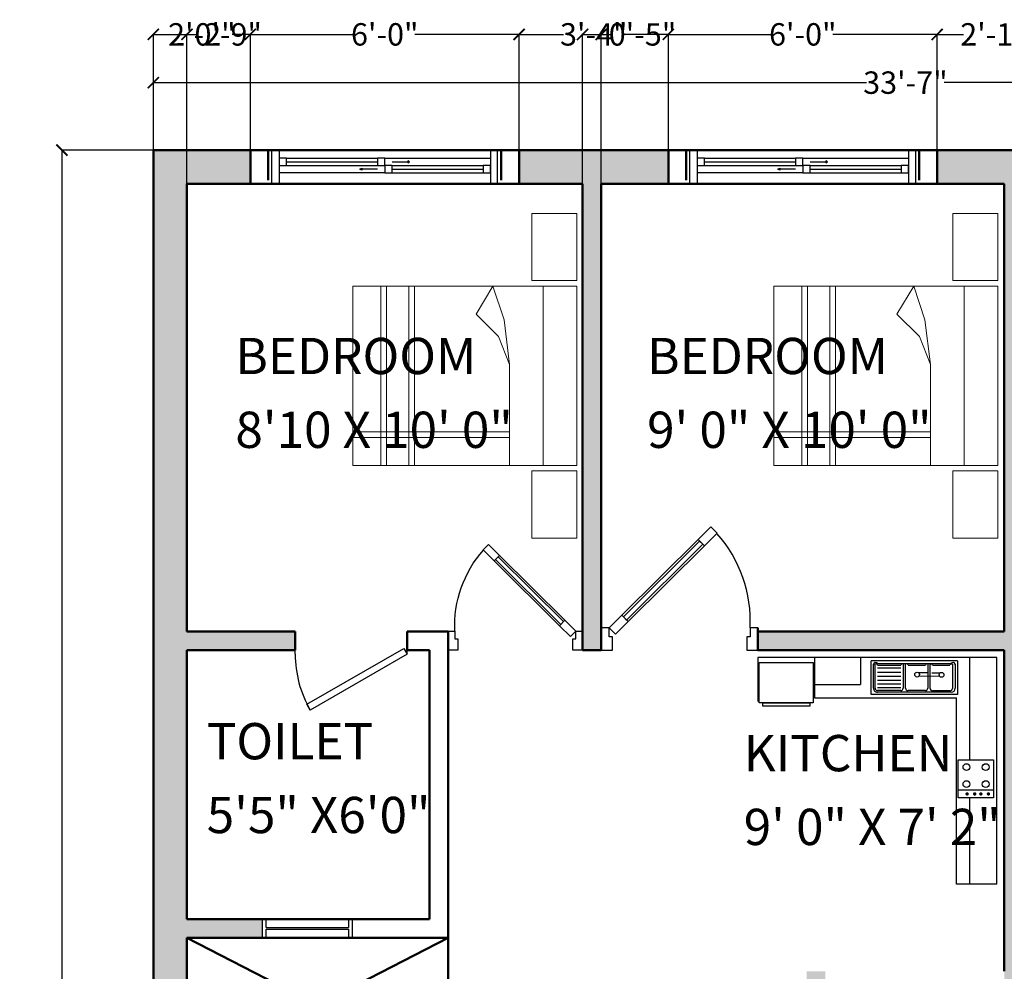
# Model space of a CAD drawing. Units: inches. Extents: x 2278 to 7495, y -71 to 1198.
# Tile 43 of 44: x 6951 to 7215, y 943 to 1198. Entities that reach past the tile are written whole.
import ezdxf

# ---------------------------------------------------------------- set-up
doc = ezdxf.new("R2010")
doc.units = ezdxf.units.IN
doc.header["$MEASUREMENT"] = 0
for name, color, linetype, lineweight in [('A-ANNO-DIMS', 2, 'Continuous', 18), ('A-AREA-IDEN', 3, 'Continuous', 18), ('A-Door', 3, 'Continuous', 25), ('A-FLOR-FIXT', 9, 'Continuous', 18), ('A-FURN', 8, 'Continuous', 18), ('A-Glaz', 4, 'Continuous', 25), ('A-Wall', 7, 'Continuous', 50), ('A-WALL-PATT', 8, 'Continuous', 18)]:
    doc.layers.add(name, color=color, linetype=linetype, lineweight=lineweight)
doc.layers.add('TEFRIŞ', color=11, linetype='Continuous')
doc.styles.get("Standard").update_dxf_attribs({"font": 'arial.ttf'})
doc.dimstyles.get("Standard").update_dxf_attribs({"dimtxt": 6, "dimasz": 3, "dimexe": 0.18, "dimexo": 0.0625, "dimgap": 0.09, "dimtad": 0, "dimtih": 1, "dimtoh": 1, "dimdec": 0, "dimzin": 0, "dimdsep": 46, "dimlunit": 3, "dimtxsty": 'Standard', "dimblk": 'ARCHTICK', "dimcen": 0.09, "dimadec": 0, "dimazin": 0, "dimtfac": 1, "dimtdec": 0, "dimtofl": 0, "dimtmove": 0, "dimatfit": 3, "dimfxl": 1, "dimtolj": 1, "dimtzin": 0, "dimarcsym": 0})

# ---------------------------------------------------------------- blocks, each defined once
blk = doc.blocks.new('A$C1DF4181C')
blk.add_lwpolyline([(120, 128), (460.7, 466.1), (432.5, 494.5), (91.8, 156.4)], close=True)
blk.add_arc((72.4, 128.7), 593.3, 357.2313, 41.4937)
at = {"layer": 'A-Door'}
for points in [[(517.5, 522.4), (460.7, 466.1), (432.5, 494.5), (489.3, 550.8)], [(63.2, 71.6), (120, 128), (91.8, 156.4), (35, 100)], [(35, 100), (0, 100), (0, 0), (50, 0), (50, 50), (50, 60), (35, 60)], [(665, 100), (665, 60), (650, 60), (650, 50), (650, 0), (700, 0), (700, 100)]]:
    blk.add_lwpolyline(points, close=True, dxfattribs=at)
at = {"layer": 'A-Glaz'}
blk.add_lwpolyline([(112.9, 135.1), (453.6, 473.2), (439.5, 487.4), (98.8, 149.3)], close=True, dxfattribs=at)
at = {"layer": 'A-Wall'}
for p, q in [((0, 0), (0, 100)), ((0, 100), (0, 0)), ((700, 0), (700, 100)), ((700, 0), (700, 100))]:
    blk.add_line(p, q, dxfattribs=at)
blk = doc.blocks.new('*U4')
for p, q in [((0, 0), (0, -6)), ((30, 0), (30, -6))]:
    blk.add_line(p, q)
blk.add_lwpolyline([(0, 0), (25.98, 15), (26.86, 13.48), (0.87, -1.52)], close=True)
blk.add_arc((0, 0), 30, 0, 30)
blk = doc.blocks.new('BED-160')
at = {"color": 0}
for p, q in [((-0.45, 2.35), (-0.45, 2.95)), ((-0.45, 2.95), (-0.05, 2.95)), ((-0.05, 2.95), (-0.05, 2.35)), ((-2.05, 2.3), (-0.05, 2.3)), ((-2.05, 0.7), (-2.05, 2.3)), ((-1.8, 0.7), (-1.8, 2.3)), ((-1.75, 0.7), (-1.75, 2.3)), ((-1.55, 0.7), (-1.55, 2.3)), ((-1.5, 0.7), (-1.5, 2.3)), ((-0.8, 2.3), (-0.95, 2.05)), ((-0.8, 2.3), (-0.7, 2)), ((-0.05, 2.35), (-0.45, 2.35)), ((-0.35, 0.7), (-0.35, 2.3)), ((-0.05, 2.3), (-0.05, 0.7)), ((-0.95, 2.05), (-0.75, 1.85)), ((-0.7, 2), (-0.65, 1.6)), ((-0.75, 1.85), (-0.65, 1.6)), ((-0.65, 1.6), (-0.65, 0.7)), ((-0.65, 1), (-2.05, 1)), ((-0.65, 0.95), (-2.05, 0.95)), ((-0.05, 0.7), (-2.05, 0.7)), ((-0.45, 0.65), (-0.05, 0.65)), ((-0.45, 0.05), (-0.45, 0.65)), ((-0.05, 0.65), (-0.05, 0.05)), ((-0.05, 0.05), (-0.45, 0.05))]:
    blk.add_line(p, q, dxfattribs=at)
blk = doc.blocks.new('A$C008029BD')
at = {"layer": 'TEFRIŞ', "ltscale": 0.05}
for p, q in [((0, 0), (0, -3.55)), ((3.37, 0), (0, 0)), ((3.37, 0), (3.37, -0.6)), ((1.522, -0.4), (0, -0.4)), ((3.37, -0.4), (2.083, -0.4)), ((0.05, -0.581), (0.05, -1.869)), ((0.05, -0.581), (0.55, -0.581)), ((0.55, -0.581), (0.55, -1.869)), ((0.086, -1.773), (0.086, -0.677)), ((0.096, -0.617), (0.454, -0.617)), ((0.099, -0.659), (0.457, -0.659)), ((0.113, -0.954), (0.113, -0.695)), ((0.493, -0.695), (0.493, -0.954)), ((0.514, -0.677), (0.514, -1.773)), ((0.6, -2.71), (0.6, -0.6)), ((3.37, -0.6), (0.6, -0.6)), ((0.23, -0.846), (0.229, -0.967)), ((0.28, -0.846), (0.277, -1.158)), ((0.096, -1.024), (0.454, -1.024)), ((0.457, -0.99), (0.099, -0.99)), ((0.228, -1.02), (0.227, -1.159)), ((0.11, -1.319), (0.11, -1.06)), ((0.49, -1.06), (0.49, -1.319)), ((0.454, -1.355), (0.096, -1.355)), ((0.096, -1.391), (0.454, -1.391)), ((0.11, -1.773), (0.11, -1.427)), ((0.154, -1.773), (0.154, -1.427)), ((0.214, -1.773), (0.214, -1.427)), ((0.274, -1.773), (0.274, -1.427)), ((0.334, -1.773), (0.334, -1.427)), ((0.39, -1.773), (0.39, -1.427)), ((0.444, -1.773), (0.444, -1.427)), ((0.49, -1.427), (0.49, -1.773)), ((0.55, -1.869), (0.05, -1.869)), ((0.454, -1.809), (0.096, -1.809)), ((0.454, -1.833), (0.096, -1.833)), ((0, -2.025), (0.4, -2.025)), ((0.4, -2.71), (0.4, -2.025)), ((0, -2.71), (0.6, -2.71)), ((0, -3.55), (0.65, -3.55))]:
    blk.add_line(p, q, dxfattribs=at)
at = {"layer": 'TEFRIŞ'}
blk.add_line((1.969, -0.05), (1.969, -0.572), dxfattribs=at)
at = {"layer": 'TEFRIŞ', "ltscale": 0.05}
for points in [[(1.522, -0.05), (2.083, -0.05), (2.083, -0.572), (1.522, -0.572)], [(0.67, -2.73), (0.67, -3.53), (0.07, -3.53), (0.07, -2.73)], [(0.72, -2.78), (0.72, -3.48), (0.67, -3.48), (0.67, -2.78)]]:
    blk.add_lwpolyline(points, close=True, dxfattribs=at)
at = {"layer": 'TEFRIŞ', "const_width": 0.025}
for points in [[(2.014, -0.123, 1), (2.039, -0.123, 1)], [(2.014, -0.236, 1), (2.039, -0.236, 1)], [(2.014, -0.327, 1), (2.039, -0.327, 1)], [(2.014, -0.44, 1), (2.039, -0.44, 1)]]:
    blk.add_lwpolyline(points, format="xyb", close=True, dxfattribs=at)
at = {"layer": 'TEFRIŞ', "ltscale": 0.05}
for centre, radius in [((1.628, -0.164), 0.0505), ((1.628, -0.45), 0.0505), ((0.255, -0.82), 0.036), ((0.252, -1.184), 0.036)]:
    blk.add_circle(centre, radius, dxfattribs=at)
at = {"layer": 'TEFRIŞ'}
for centre in [(1.88, -0.164), (1.88, -0.45)]:
    blk.add_circle(centre, 0.0505, dxfattribs=at)
at = {"layer": 'TEFRIŞ', "ltscale": 0.05}
for centre, radius, start, end in [((0.108, -0.649), 0.0351, 110.4976, 230.5777), ((0.118, -0.673), 0.023, 143.9853, 258.5157), ((0.454, -0.677), 0.06, 0, 90), ((0.457, -0.695), 0.036, 0, 90), ((0.115, -1.038), 0.023, 143.9853, 258.5157), ((0.118, -0.976), 0.023, 101.4843, 216.0147), ((0.454, -1.06), 0.036, 0, 90), ((0.457, -0.954), 0.036, 270, 0), ((0.115, -1.341), 0.023, 101.4843, 216.0147), ((0.115, -1.405), 0.023, 143.9853, 258.5157), ((0.454, -1.319), 0.036, 270, 0), ((0.454, -1.427), 0.036, 0, 90), ((0.108, -1.801), 0.0351, 129.4223, 249.5024), ((0.115, -1.796), 0.023, 101.4843, 216.0147), ((0.454, -1.773), 0.06, 270, 0), ((0.454, -1.773), 0.036, 270, 0)]:
    blk.add_arc(centre, radius, start, end, dxfattribs=at)
blk = doc.blocks.new('_ArchTick')
at = {"color": 0, "linetype": 'ByBlock', "const_width": 0.15}
blk.add_lwpolyline([(-0.5, -0.5), (0.5, 0.5)], dxfattribs=at)
blk = doc.blocks.new('*D27')
at = {"layer": 'A-ANNO-DIMS', "color": 0, "lineweight": -2, "transparency": 16777216}
for p, q in [((6987.05, 1163.47), (6962.44, 1163.47)), ((6962.62, 1163.47), (6962.62, 940.12)), ((6962.62, 710.47), (6962.62, 933.81)), ((6987.05, 710.47), (6962.44, 710.47))]:
    blk.add_line(p, q, dxfattribs=at)
at = {"layer": 'Defpoints', "color": 0, "transparency": 16777216}
for p in [(6987.12, 1163.47), (6962.62, 710.47), (6987.12, 710.47)]:
    blk.add_point(p, dxfattribs=at)
at = {"layer": 'A-ANNO-DIMS', "color": 0, "lineweight": -2, "transparency": 16777216, "xscale": 3, "yscale": 3, "zscale": 3}
for p, rotation in [((6962.62, 1163.47), 90), ((6962.62, 710.47), 270)]:
    blk.add_blockref('_ArchTick', p, dxfattribs=dict(at, rotation=rotation))
at = {"layer": 'A-ANNO-DIMS', "color": 0, "transparency": 16777216, "insert": (6962.62, 936.97), "char_height": 6, "attachment_point": 5}
blk.add_mtext('\\A1;37\'-9"', dxfattribs=at)
blk = doc.blocks.new('*D28')
at = {"layer": 'A-ANNO-DIMS', "color": 0, "lineweight": -2, "transparency": 16777216}
for p, q in [((6987.12, 1163.53), (6987.12, 1181.72)), ((6987.12, 1181.54), (7178.22, 1181.54)), ((7390.12, 1181.54), (7199.01, 1181.54)), ((7390.12, 1163.53), (7390.12, 1181.72))]:
    blk.add_line(p, q, dxfattribs=at)
at = {"layer": 'Defpoints', "color": 0, "transparency": 16777216}
for p in [(7390.12, 1181.54), (6987.12, 1163.47), (7390.12, 1163.47)]:
    blk.add_point(p, dxfattribs=at)
at = {"layer": 'A-ANNO-DIMS', "color": 0, "lineweight": -2, "transparency": 16777216, "xscale": 3, "yscale": 3, "zscale": 3, "rotation": 180}
blk.add_blockref('_ArchTick', (6987.12, 1181.54), dxfattribs=at)
at = {"layer": 'A-ANNO-DIMS', "color": 0, "lineweight": -2, "transparency": 16777216, "xscale": 3, "yscale": 3, "zscale": 3}
blk.add_blockref('_ArchTick', (7390.12, 1181.54), dxfattribs=at)
at = {"layer": 'A-ANNO-DIMS', "color": 0, "transparency": 16777216, "insert": (7188.62, 1181.54), "char_height": 6, "attachment_point": 5}
blk.add_mtext('\\A1;33\'-7"', dxfattribs=at)
blk = doc.blocks.new('*D93')
at = {"layer": 'A-ANNO-DIMS', "color": 0, "lineweight": -2, "transparency": 16777216}
for p, q in [((6987.12, 1163.53), (6987.12, 1194.65)), ((6987.12, 1194.47), (6992, 1194.47)), ((7013.12, 1194.47), (7008.23, 1194.47)), ((7013.12, 1163.53), (7013.12, 1194.65))]:
    blk.add_line(p, q, dxfattribs=at)
at = {"layer": 'Defpoints', "color": 0, "transparency": 16777216}
for p in [(7013.12, 1194.47), (6987.12, 1163.47), (7013.12, 1163.47)]:
    blk.add_point(p, dxfattribs=at)
at = {"layer": 'A-ANNO-DIMS', "color": 0, "lineweight": -2, "transparency": 16777216, "xscale": 3, "yscale": 3, "zscale": 3, "rotation": 180}
blk.add_blockref('_ArchTick', (6987.12, 1194.47), dxfattribs=at)
at = {"layer": 'A-ANNO-DIMS', "color": 0, "lineweight": -2, "transparency": 16777216, "xscale": 3, "yscale": 3, "zscale": 3}
blk.add_blockref('_ArchTick', (7013.12, 1194.47), dxfattribs=at)
at = {"layer": 'A-ANNO-DIMS', "color": 0, "transparency": 16777216, "insert": (7000.12, 1194.47), "char_height": 6, "attachment_point": 5}
blk.add_mtext('\\A1;2\'-2"', dxfattribs=at)
blk = doc.blocks.new('*D94')
at = {"layer": 'A-ANNO-DIMS', "color": 0, "lineweight": -2, "transparency": 16777216}
for p, q in [((7013.12, 1163.53), (7013.12, 1194.65)), ((7013.12, 1194.47), (7041.03, 1194.47)), ((7085.12, 1194.47), (7057.2, 1194.47)), ((7085.12, 1163.53), (7085.12, 1194.65))]:
    blk.add_line(p, q, dxfattribs=at)
at = {"layer": 'Defpoints', "color": 0, "transparency": 16777216}
for p in [(7085.12, 1194.47), (7013.12, 1163.47), (7085.12, 1163.47)]:
    blk.add_point(p, dxfattribs=at)
at = {"layer": 'A-ANNO-DIMS', "color": 0, "lineweight": -2, "transparency": 16777216, "xscale": 3, "yscale": 3, "zscale": 3, "rotation": 180}
blk.add_blockref('_ArchTick', (7013.12, 1194.47), dxfattribs=at)
at = {"layer": 'A-ANNO-DIMS', "color": 0, "lineweight": -2, "transparency": 16777216, "xscale": 3, "yscale": 3, "zscale": 3}
blk.add_blockref('_ArchTick', (7085.12, 1194.47), dxfattribs=at)
at = {"layer": 'A-ANNO-DIMS', "color": 0, "transparency": 16777216, "insert": (7049.12, 1194.47), "char_height": 6, "attachment_point": 5}
blk.add_mtext('\\A1;6\'-0"', dxfattribs=at)
blk = doc.blocks.new('*D95')
at = {"layer": 'A-ANNO-DIMS', "color": 0, "lineweight": -2, "transparency": 16777216}
for p, q in [((7085.12, 1163.53), (7085.12, 1194.65)), ((7085.12, 1194.47), (7097.05, 1194.47)), ((7125.12, 1194.47), (7113.18, 1194.47)), ((7125.12, 1163.53), (7125.12, 1194.65))]:
    blk.add_line(p, q, dxfattribs=at)
at = {"layer": 'Defpoints', "color": 0, "transparency": 16777216}
for p in [(7125.12, 1194.47), (7085.12, 1163.47), (7125.12, 1163.47)]:
    blk.add_point(p, dxfattribs=at)
at = {"layer": 'A-ANNO-DIMS', "color": 0, "lineweight": -2, "transparency": 16777216, "xscale": 3, "yscale": 3, "zscale": 3, "rotation": 180}
blk.add_blockref('_ArchTick', (7085.12, 1194.47), dxfattribs=at)
at = {"layer": 'A-ANNO-DIMS', "color": 0, "lineweight": -2, "transparency": 16777216, "xscale": 3, "yscale": 3, "zscale": 3}
blk.add_blockref('_ArchTick', (7125.12, 1194.47), dxfattribs=at)
at = {"layer": 'A-ANNO-DIMS', "color": 0, "transparency": 16777216, "insert": (7105.12, 1194.47), "char_height": 6, "attachment_point": 5}
blk.add_mtext('\\A1;3\'-4"', dxfattribs=at)
blk = doc.blocks.new('*D96')
at = {"layer": 'A-ANNO-DIMS', "color": 0, "lineweight": -2, "transparency": 16777216}
for p, q in [((7125.12, 1163.53), (7125.12, 1194.65)), ((7125.12, 1194.47), (7153.03, 1194.47)), ((7197.12, 1194.47), (7169.2, 1194.47)), ((7197.12, 1163.53), (7197.12, 1194.65))]:
    blk.add_line(p, q, dxfattribs=at)
at = {"layer": 'Defpoints', "color": 0, "transparency": 16777216}
for p in [(7197.12, 1194.47), (7125.12, 1163.47), (7197.12, 1163.47)]:
    blk.add_point(p, dxfattribs=at)
at = {"layer": 'A-ANNO-DIMS', "color": 0, "lineweight": -2, "transparency": 16777216, "xscale": 3, "yscale": 3, "zscale": 3, "rotation": 180}
blk.add_blockref('_ArchTick', (7125.12, 1194.47), dxfattribs=at)
at = {"layer": 'A-ANNO-DIMS', "color": 0, "lineweight": -2, "transparency": 16777216, "xscale": 3, "yscale": 3, "zscale": 3}
blk.add_blockref('_ArchTick', (7197.12, 1194.47), dxfattribs=at)
at = {"layer": 'A-ANNO-DIMS', "color": 0, "transparency": 16777216, "insert": (7161.12, 1194.47), "char_height": 6, "attachment_point": 5}
blk.add_mtext('\\A1;6\'-0"', dxfattribs=at)
blk = doc.blocks.new('*D97')
at = {"layer": 'A-ANNO-DIMS', "color": 0, "lineweight": -2, "transparency": 16777216}
for p, q in [((7197.12, 1163.53), (7197.12, 1194.65)), ((7197.12, 1194.47), (7204.17, 1194.47)), ((7232.12, 1194.47), (7225.06, 1194.47)), ((7232.12, 1163.53), (7232.12, 1194.65))]:
    blk.add_line(p, q, dxfattribs=at)
at = {"layer": 'Defpoints', "color": 0, "transparency": 16777216}
for p in [(7232.12, 1194.47), (7197.12, 1163.47), (7232.12, 1163.47)]:
    blk.add_point(p, dxfattribs=at)
at = {"layer": 'A-ANNO-DIMS', "color": 0, "lineweight": -2, "transparency": 16777216, "xscale": 3, "yscale": 3, "zscale": 3, "rotation": 180}
blk.add_blockref('_ArchTick', (7197.12, 1194.47), dxfattribs=at)
at = {"layer": 'A-ANNO-DIMS', "color": 0, "lineweight": -2, "transparency": 16777216, "xscale": 3, "yscale": 3, "zscale": 3}
blk.add_blockref('_ArchTick', (7232.12, 1194.47), dxfattribs=at)
at = {"layer": 'A-ANNO-DIMS', "color": 0, "transparency": 16777216, "insert": (7214.62, 1194.47), "char_height": 6, "attachment_point": 5}
blk.add_mtext('\\A1;2\'-11"', dxfattribs=at)
blk = doc.blocks.new('*D102')
at = {"layer": 'A-ANNO-DIMS', "color": 0, "lineweight": -2, "transparency": 16777216}
for p, q in [((6987.12, 1163.53), (6987.12, 1194.65)), ((6987.12, 1194.47), (6996.12, 1194.47)), ((6996.12, 1154.53), (6996.12, 1194.65)), ((6996.12, 1194.47), (6999.12, 1194.47))]:
    blk.add_line(p, q, dxfattribs=at)
at = {"layer": 'Defpoints', "color": 0, "transparency": 16777216}
for p in [(6996.12, 1194.47), (6987.12, 1163.47), (6996.12, 1154.47)]:
    blk.add_point(p, dxfattribs=at)
at = {"layer": 'A-ANNO-DIMS', "color": 0, "lineweight": -2, "transparency": 16777216, "xscale": 3, "yscale": 3, "zscale": 3, "rotation": 180}
blk.add_blockref('_ArchTick', (6987.12, 1194.47), dxfattribs=at)
at = {"layer": 'A-ANNO-DIMS', "color": 0, "lineweight": -2, "transparency": 16777216, "xscale": 3, "yscale": 3, "zscale": 3}
blk.add_blockref('_ArchTick', (6996.12, 1194.47), dxfattribs=at)
at = {"layer": 'A-ANNO-DIMS', "color": 0, "transparency": 16777216, "insert": (7007.18, 1194.47), "char_height": 6, "attachment_point": 5}
blk.add_mtext('\\A1;0\'-9"', dxfattribs=at)
blk = doc.blocks.new('*D103')
at = {"layer": 'A-ANNO-DIMS', "color": 0, "lineweight": -2, "transparency": 16777216}
for p, q in [((7102.12, 1029.53), (7102.12, 1194.65)), ((7102.12, 1194.47), (7107.12, 1194.47)), ((7107.12, 1029.53), (7107.12, 1194.65)), ((7107.12, 1194.47), (7110.12, 1194.47))]:
    blk.add_line(p, q, dxfattribs=at)
at = {"layer": 'Defpoints', "color": 0, "transparency": 16777216}
for p in [(7107.12, 1194.47), (7102.12, 1029.47), (7107.12, 1029.47)]:
    blk.add_point(p, dxfattribs=at)
at = {"layer": 'A-ANNO-DIMS', "color": 0, "lineweight": -2, "transparency": 16777216, "xscale": 3, "yscale": 3, "zscale": 3, "rotation": 180}
blk.add_blockref('_ArchTick', (7102.12, 1194.47), dxfattribs=at)
at = {"layer": 'A-ANNO-DIMS', "color": 0, "lineweight": -2, "transparency": 16777216, "xscale": 3, "yscale": 3, "zscale": 3}
blk.add_blockref('_ArchTick', (7107.12, 1194.47), dxfattribs=at)
at = {"layer": 'A-ANNO-DIMS', "color": 0, "transparency": 16777216, "insert": (7118.18, 1194.47), "char_height": 6, "attachment_point": 5}
blk.add_mtext('\\A1;0\'-5"', dxfattribs=at)

msp = doc.modelspace()

# ---------------------------------------------------------------- hatches: boundary and pattern name
at = {"layer": 'A-WALL-PATT'}
h = msp.add_hatch(dxfattribs=at)
h.set_pattern_fill('ANSI36', color=256, scale=30)
h.set_pattern_definition([(45, (4673.2453, 0), (1.988738, 7.2920387), [9.375, -1.875, 0, -1.875])])
h.paths.add_polyline_path([(7016.37, 957.47), (6996.12, 957.47), (6996.12, 1029.47), (7025.12, 1029.47), (7025.12, 1034.47), (6996.12, 1034.47), (6996.12, 1154.47), (7013.12, 1154.47), (7013.12, 1163.47), (6987.12, 1163.47), (6987.12, 710.47), (7119.12, 710.47), (7119.12, 719.47), (6996.12, 719.47), (6996.12, 807.47), (7078.12, 807.47), (7078.12, 812.47), (7066.12, 812.47), (7066.12, 881.47), (7061.12, 881.47), (7061.12, 812.47), (6996.12, 812.47), (6996.12, 911.47), (7019.12, 911.47), (7019.12, 916.47), (6996.12, 916.47), (6996.12, 952.47), (7016.37, 952.47)])
h.paths.add_polyline_path([(7125.12, 1163.47), (7085.12, 1163.47), (7085.12, 1154.47), (7102.12, 1154.47), (7102.12, 1034.47), (7102.12, 1029.47), (7107.12, 1029.47), (7107.12, 1154.47), (7125.12, 1154.47)])
h.paths.add_polyline_path([(7232.12, 1163.47), (7197.12, 1163.47), (7197.12, 1154.47), (7215.12, 1154.47), (7215.12, 1034.47), (7149.12, 1034.47), (7149.12, 1029.47), (7215.12, 1029.47), (7215.12, 943.47), (7215.12, 940.13), (7215.12, 876.47), (7167.12, 876.47), (7167.12, 943.47), (7162.12, 943.47), (7162.12, 871.47), (7162.12, 865.74), (7167.12, 865.74), (7167.12, 871.47), (7215.12, 871.47), (7215.12, 805.47), (7220.12, 805.47), (7220.12, 1077.47), (7232.12, 1077.47), (7232.12, 1082.47), (7220.12, 1082.47), (7220.12, 1154.47), (7232.12, 1154.47)])
h.paths.add_polyline_path([(7390.12, 937.97), (7381.12, 937.97), (7381.12, 911.47), (7268.12, 911.47), (7268.12, 906.47), (7381.12, 906.47), (7381.12, 869.47), (7390.12, 869.47)])
h.paths.add_polyline_path([(7390.12, 1163.47), (7363.12, 1163.47), (7363.12, 1154.47), (7381.12, 1154.47), (7381.12, 1041.47), (7268.12, 1041.47), (7268.12, 1036.47), (7381.12, 1036.47), (7381.12, 1009.97), (7390.12, 1009.97)])
h.paths.add_polyline_path([(7291.12, 1163.47), (7256.12, 1163.47), (7256.12, 1154.47), (7268.12, 1154.47), (7268.12, 1082.47), (7262.12, 1082.47), (7262.12, 1077.47), (7273.12, 1077.47), (7273.12, 1154.47), (7291.12, 1154.47)])
h.paths.add_polyline_path([(7390.12, 797.47), (7381.12, 797.47), (7381.12, 760.47), (7336.62, 760.47), (7336.62, 755.47), (7390.12, 755.47)])
h.paths.add_polyline_path([(7264.62, 760.47), (7220.12, 760.47), (7220.12, 763.47), (7215.12, 763.47), (7215.12, 755.47), (7264.62, 755.47)])

# ---------------------------------------------------------------- linework, layer by layer
at = {"layer": 'A-Glaz'}
for p, q in [((7020.82, 1163.47), (7077.41, 1163.47)), ((7132.82, 1163.47), (7189.41, 1163.47)), ((7022.77, 1161.3), (7047.16, 1161.3)), ((7049.12, 1161.3), (7077.41, 1161.3)), ((7134.77, 1161.3), (7159.16, 1161.3)), ((7161.12, 1161.3), (7189.41, 1161.3)), ((7022.77, 1160.32), (7047.16, 1160.32)), ((7022.77, 1159.35), (7047.16, 1159.35)), ((7047.16, 1158.37), (7042.97, 1158.37)), ((7051.07, 1160.32), (7055.26, 1160.32)), ((7051.07, 1159.35), (7075.46, 1159.35)), ((7051.07, 1158.37), (7075.46, 1158.37)), ((7134.77, 1160.32), (7159.16, 1160.32)), ((7134.77, 1159.35), (7159.16, 1159.35)), ((7159.16, 1158.37), (7154.97, 1158.37)), ((7163.07, 1160.32), (7167.26, 1160.32)), ((7163.07, 1159.35), (7187.46, 1159.35)), ((7163.07, 1158.37), (7187.46, 1158.37)), ((7049.12, 1157.39), (7020.82, 1157.39)), ((7051.07, 1157.39), (7075.46, 1157.39)), ((7161.12, 1157.39), (7132.82, 1157.39)), ((7163.07, 1157.39), (7187.46, 1157.39)), ((7020.82, 1154.47), (7077.41, 1154.47)), ((7132.82, 1154.47), (7189.41, 1154.47)), ((7016.37, 957.47), (7040.37, 957.47)), ((7016.37, 952.47), (7016.37, 957.47)), ((7017.37, 955.17), (7017.37, 957.47)), ((7017.37, 955.17), (7039.37, 955.17)), ((7039.37, 957.47), (7039.37, 955.17)), ((7040.37, 957.47), (7040.37, 952.47)), ((7040.37, 952.47), (7016.37, 952.47)), ((7017.37, 952.47), (7017.37, 954.77)), ((7017.37, 954.77), (7039.37, 954.77)), ((7039.37, 954.77), (7039.37, 952.47))]:
    msp.add_line(p, q, dxfattribs=at)
for points in [[(7020.82, 1154.47), (7018.86, 1154.47), (7018.86, 1163.47), (7020.82, 1163.47)], [(7077.41, 1154.47), (7079.37, 1154.47), (7079.37, 1163.47), (7077.41, 1163.47)], [(7132.82, 1154.47), (7130.86, 1154.47), (7130.86, 1163.47), (7132.82, 1163.47)], [(7189.41, 1154.47), (7191.37, 1154.47), (7191.37, 1163.47), (7189.41, 1163.47)], [(7020.82, 1159.35), (7022.77, 1159.35), (7022.77, 1161.3), (7020.82, 1161.3)], [(7047.16, 1159.35), (7049.12, 1159.35), (7049.12, 1161.3), (7047.16, 1161.3)], [(7132.82, 1159.35), (7134.77, 1159.35), (7134.77, 1161.3), (7132.82, 1161.3)], [(7159.16, 1159.35), (7161.12, 1159.35), (7161.12, 1161.3), (7159.16, 1161.3)], [(7042.47, 1158.37), (7042.97, 1158.66), (7042.97, 1158.08)], [(7049.12, 1157.39), (7051.07, 1157.39), (7051.07, 1159.35), (7049.12, 1159.35)], [(7055.76, 1160.32), (7055.26, 1160.61), (7055.26, 1160.03)], [(7075.46, 1157.39), (7077.41, 1157.39), (7077.41, 1159.35), (7075.46, 1159.35)], [(7154.47, 1158.37), (7154.97, 1158.66), (7154.97, 1158.08)], [(7161.12, 1157.39), (7163.07, 1157.39), (7163.07, 1159.35), (7161.12, 1159.35)], [(7167.76, 1160.32), (7167.26, 1160.61), (7167.26, 1160.03)], [(7187.46, 1157.39), (7189.41, 1157.39), (7189.41, 1159.35), (7187.46, 1159.35)]]:
    msp.add_lwpolyline(points, close=True, dxfattribs=at)
at = {"layer": 'A-Wall'}
for p, q in [((6987.12, 1163.47), (6987.12, 710.47)), ((6987.12, 1163.47), (7390.12, 1163.47)), ((7013.12, 1154.47), (7013.12, 1163.47)), ((7018.86, 1163.47), (7013.12, 1163.47)), ((7079.37, 1163.47), (7085.12, 1163.47)), ((7085.12, 1154.47), (7085.12, 1163.47)), ((7125.12, 1154.47), (7125.12, 1163.47)), ((7130.86, 1163.47), (7125.12, 1163.47)), ((7191.37, 1163.47), (7197.12, 1163.47)), ((7197.12, 1154.47), (7197.12, 1163.47)), ((7017.89, 1163.25), (7017.89, 1155.44)), ((7080.34, 1163.25), (7080.34, 1155.44)), ((7129.89, 1163.25), (7129.89, 1155.44)), ((7192.34, 1163.25), (7192.34, 1155.44)), ((6996.12, 1154.47), (6996.12, 1034.47)), ((6996.12, 1154.47), (7102.12, 1154.47)), ((7018.86, 1154.47), (7013.12, 1154.47)), ((7079.37, 1154.47), (7085.12, 1154.47)), ((7102.12, 1154.47), (7102.12, 1034.47)), ((7107.12, 1154.47), (7107.12, 1029.47)), ((7107.12, 1154.47), (7215.12, 1154.47)), ((7130.86, 1154.47), (7125.12, 1154.47)), ((7191.37, 1154.47), (7197.12, 1154.47)), ((7215.12, 1154.47), (7215.12, 1034.47)), ((6996.12, 1034.47), (7025.12, 1034.47)), ((7025.12, 1029.47), (7025.12, 1034.47)), ((7055.12, 1034.47), (7066.12, 1034.47)), ((7055.12, 1029.47), (7055.12, 1034.47)), ((7066.12, 1034.47), (7066.12, 1029.47)), ((7102.12, 1034.47), (7102.12, 1029.47)), ((7149.12, 1034.47), (7215.12, 1034.47)), ((7149.12, 1029.47), (7149.12, 1034.47)), ((6996.12, 1029.47), (6996.12, 957.47)), ((6996.12, 1029.47), (7025.12, 1029.47)), ((7055.12, 1029.47), (7061.12, 1029.47)), ((7061.12, 1029.47), (7061.12, 957.47)), ((7066.12, 1029.47), (7066.12, 911.47)), ((7102.12, 1029.47), (7107.12, 1029.47)), ((7149.12, 1029.47), (7215.12, 1029.47)), ((7215.12, 1029.47), (7215.12, 943.47)), ((6996.12, 957.47), (7061.12, 957.47)), ((6996.12, 952.47), (6996.12, 916.47)), ((6996.12, 952.47), (7066.12, 952.47)), ((7066.12, 916.47), (6996.12, 952.47)), ((6996.12, 916.47), (7066.12, 952.47))]:
    msp.add_line(p, q, dxfattribs=at)

# ---------------------------------------------------------------- block references
at = {"layer": 'A-Door'}
for p, xscale, yscale, zscale in [((7107.12, 1029.47), 0.0599999999999766, 0.0599999999999766, 0.0599999999999766), ((7102.12, 1029.47), -0.051428571401403, 0.051428571401403, 0.051428571401403)]:
    msp.add_blockref('A$C1DF4181C', p, dxfattribs=dict(at, xscale=xscale, yscale=yscale, zscale=zscale))
at = {"layer": 'A-Door', "rotation": 180}
msp.add_blockref('*U4', (7055.12, 1028.47), dxfattribs=at)
at = {"layer": 'A-FLOR-FIXT', "xscale": 18.01737512370223, "yscale": 18.01737512370223, "zscale": 18.01737512370223, "rotation": 270}
msp.add_blockref('A$C008029BD', (7213.08, 1027.5), dxfattribs=at)
at = {"layer": 'A-FURN', "xscale": 29.9999999999997, "yscale": 29.9999999999997, "zscale": 29.9999999999997}
for p in [(7102.07, 1058), (7214.85, 1058)]:
    msp.add_blockref('BED-160', p, dxfattribs=at)

# ---------------------------------------------------------------- texts
at = {"layer": 'A-AREA-IDEN'}
for s, height, p in [('BEDROOM', 9.72, (7009.1, 1103.45)), ('BEDROOM', 9.72, (7119.41, 1103.45)), ('8\'10 X 10\' 0"', 9.7203, (7009.1, 1083.68)), ('9\' 0" X 10\' 0"', 9.7203, (7119.41, 1083.68)), ('TOILET', 9.72, (7001.42, 1000.25)), ('KITCHEN', 9.72, (7145.3, 997.06)), ('5\'5" X6\'0"', 9.72, (7001.42, 980.48)), ('9\' 0" X 7\' 2"', 9.7203, (7145.3, 977.29))]:
    msp.add_text(s, height=height, dxfattribs=at).set_placement(p)

# ---------------------------------------------------------------- dimensions: what is measured, and where the dimension line sits
at = {"layer": 'A-ANNO-DIMS'}
for base, p1, p2, override, picture, middle in [((7013.12, 1194.47), (6987.12, 1163.47), (7013.12, 1163.47), {"dimdec": 1, "dimlfac": 1, "dimrnd": 0, "dimzin": 1, "dimdsep": 46, "dimlunit": 4, "dimfrac": 2}, '*D93', (7000.12, 1194.47)), ((6996.12, 1194.47), (6987.12, 1163.47), (6996.12, 1154.47), {"dimdec": 1, "dimlfac": 1, "dimrnd": 0, "dimzin": 1, "dimdsep": 46, "dimlunit": 4, "dimfrac": 2}, '*D102', (7007.18, 1194.47)), ((7085.12, 1194.47), (7013.12, 1163.47), (7085.12, 1163.47), {"dimdec": 1, "dimlfac": 1, "dimrnd": 0, "dimzin": 1, "dimdsep": 46, "dimlunit": 4, "dimfrac": 2}, '*D94', (7049.12, 1194.47)), ((7125.12, 1194.47), (7085.12, 1163.47), (7125.12, 1163.47), {"dimdec": 1, "dimlfac": 1, "dimrnd": 0, "dimzin": 1, "dimdsep": 46, "dimlunit": 4, "dimfrac": 2}, '*D95', (7105.12, 1194.47)), ((7107.12, 1194.47), (7102.12, 1029.47), (7107.12, 1029.47), {"dimdec": 1, "dimlfac": 1, "dimrnd": 0, "dimzin": 1, "dimdsep": 46, "dimlunit": 4, "dimfrac": 2}, '*D103', (7118.18, 1194.47)), ((7197.12, 1194.47), (7125.12, 1163.47), (7197.12, 1163.47), {"dimdec": 1, "dimlfac": 1, "dimrnd": 0, "dimzin": 1, "dimdsep": 46, "dimlunit": 4, "dimfrac": 2}, '*D96', (7161.12, 1194.47)), ((7232.12, 1194.47), (7197.12, 1163.47), (7232.12, 1163.47), {"dimdec": 1, "dimlfac": 1, "dimrnd": 0, "dimzin": 1, "dimdsep": 46, "dimlunit": 4, "dimfrac": 2}, '*D97', (7214.62, 1194.47)), ((7390.12, 1181.54), (6987.12, 1163.47), (7390.12, 1163.47), {"dimclrd": 0, "dimclre": 0, "dimclrt": 0}, '*D28', (7188.62, 1181.54))]:
    dim = msp.add_linear_dim(base=base, p1=p1, p2=p2, dimstyle='Standard', override=override, dxfattribs=at)
    dim.commit()
    dim.dimension.update_dxf_attribs({"geometry": picture, "text_midpoint": middle})
dim = msp.add_linear_dim(base=(6962.62, 710.47), p1=(6987.12, 1163.47), p2=(6987.12, 710.47), angle=90, dimstyle='Standard', override={"dimclrd": 0, "dimclre": 0, "dimclrt": 0}, dxfattribs=at)
dim.commit()
dim.dimension.update_dxf_attribs({"geometry": '*D27', "text_midpoint": (6962.62, 936.97)})

doc.saveas('drawing.dxf')
